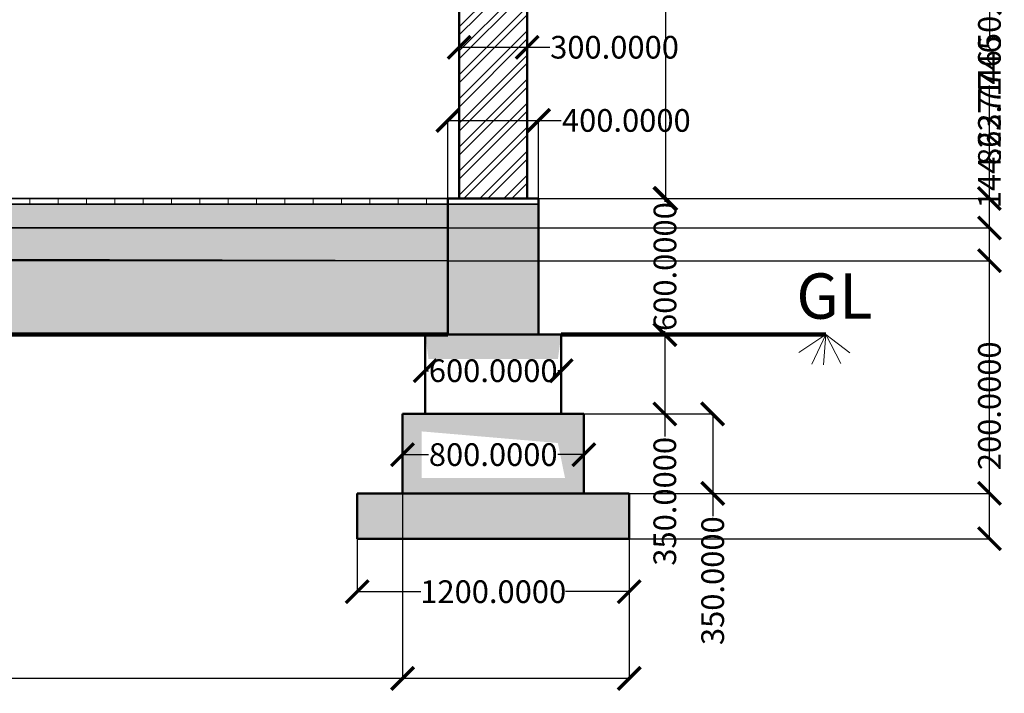
# Model space of a CAD drawing. Units: millimetres. Extents: x -4055 to 12299, y -682 to 5380.
# Tile 3 of 4: x 7955 to 12299, y -682 to 2289. Entities that reach past the tile are written whole.
import ezdxf

# ---------------------------------------------------------------- set-up
doc = ezdxf.new("R2010")
doc.units = ezdxf.units.MM
doc.header["$MEASUREMENT"] = 0
for name, color, linetype, lineweight in [('A-ANNO-DIMS', 2, 'Continuous', 18), ('A-ANNO-SYMB', 18, 'Continuous', 18), ('A-ANNO-TEXT', 7, 'Continuous', 18), ('A-FLOR', 7, 'Continuous', 35), ('A-FLOR-PATT', 8, 'Continuous', 13), ('A-WALL', 7, 'Continuous', 50), ('A-WALL-PATT', 8, 'Continuous', 13), ('gl', 18, 'Continuous', 120), ('S-FNDN', 7, 'Continuous', 50), ('S-FNDN-PATT', 8, 'Continuous', 13)]:
    doc.layers.add(name, color=color, linetype=linetype, lineweight=lineweight)
doc.styles.get("Standard").update_dxf_attribs({"font": 'arial.ttf'})
doc.dimstyles.get("Standard").update_dxf_attribs({"dimtxt": 100, "dimasz": 100, "dimexe": 0.18, "dimexo": 0.0625, "dimgap": 0.09, "dimtad": 0, "dimdec": 4, "dimzin": 0, "dimdsep": 46, "dimtxsty": 'Standard', "dimblk": 'ARCHTICK', "dimcen": 0.09, "dimclrd": 3, "dimclre": 6, "dimclrt": 1, "dimadec": 0, "dimazin": 0, "dimtfac": 1, "dimtdec": 4, "dimtofl": 0, "dimtmove": 0, "dimatfit": 3, "dimfxl": 1, "dimtolj": 1, "dimtzin": 0, "dimlwd": 30, "dimarcsym": 0})
pattern_1 = [(50, (0, 0), (71.72602, -6.2752), [7.5, -82.5]), (355, (0, 0), (-13.87513, 75.2192), [6, -66]), (100.45144, (5.98, -0.52), (57.8509, 68.944), [6.374, -70.1142]), (46.1842, (0, 20), (106.7241, -16.5519), [11.25, -123.75]), (96.6356, (8.89, 18.62), (93.4662, 97.4119), [9.561, -105.1714]), (351.1842, (0, 20), (93.4662, 97.4119), [9, -99]), (21, (10, 15), (59.6907, -40.2619), [7.5, -82.5]), (326, (10, 15), (24.33153, 72.515), [6, -66]), (71.45144, (14.974, 11.645), (84.02224, 32.2531), [6.374, -70.1142]), (37.5, (0, 0), (1.215986, 33.289385), [0, -65.2, 0, -67, 0, -66.25]), (7.5, (0, 0), (26.30695, 39.44117), [0, -38.2, 0, -63.7, 0, -25.25]), (327.5, (-22.3, 0), (53.382244, -2.25549), [0, -25, 0, -78, 0, -103.5]), (317.5, (-32.3, 0), (58.31862, 10.0105), [0, -32.5, 0, -51.8, 0, -73.5])]

# ---------------------------------------------------------------- blocks, each defined once
blk = doc.blocks.new('_ArchTick')
at = {"color": 0, "linetype": 'ByBlock', "const_width": 0.15}
blk.add_lwpolyline([(-0.5, -0.5), (0.5, 0.5)], dxfattribs=at)
blk = doc.blocks.new('*D2')
at = {"layer": 'A-ANNO-DIMS', "color": 0, "lineweight": -2, "transparency": 16777216}
for p, q in [((10194.1, 4500), (10805.3, 4500)), ((10194.1, 1500), (10805.3, 1500))]:
    blk.add_line(p, q, dxfattribs=at)
at = {"layer": 'A-ANNO-DIMS', "color": 0, "lineweight": 30, "transparency": 16777216}
for p, q in [((10805.2, 4500), (10805.2, 3324)), ((10805.2, 1500), (10805.2, 2676))]:
    blk.add_line(p, q, dxfattribs=at)
at = {"layer": 'Defpoints', "color": 0, "transparency": 16777216}
for p in [(10194, 4500), (10194, 1500), (10805.2, 1500)]:
    blk.add_point(p, dxfattribs=at)
at = {"layer": 'A-ANNO-DIMS', "color": 0, "lineweight": 30, "transparency": 16777216, "xscale": 100, "yscale": 100, "zscale": 100}
for p, rotation in [((10805.2, 4500), 90), ((10805.2, 1500), 270)]:
    blk.add_blockref('_ArchTick', p, dxfattribs=dict(at, rotation=rotation))
at = {"layer": 'A-ANNO-DIMS', "color": 0, "transparency": 16777216, "insert": (10805.2, 3000), "char_height": 100, "attachment_point": 5, "rotation": 90}
blk.add_mtext('\\A1;3000.0000', dxfattribs=at)
blk = doc.blocks.new('*D3')
at = {"layer": 'A-ANNO-DIMS', "color": 0, "lineweight": -2, "transparency": 16777216}
for p, q in [((10194.1, 1500), (10801.7, 1500)), ((10194.1, 900), (10801.7, 900))]:
    blk.add_line(p, q, dxfattribs=at)
at = {"layer": 'A-ANNO-DIMS', "color": 0, "lineweight": 30, "transparency": 16777216}
for p, q in [((10801.6, 1500), (10801.6, 1485.5)), ((10801.6, 900), (10801.6, 914.5))]:
    blk.add_line(p, q, dxfattribs=at)
at = {"layer": 'Defpoints', "color": 0, "transparency": 16777216}
for p in [(10194, 1500), (10194, 900), (10801.6, 900)]:
    blk.add_point(p, dxfattribs=at)
at = {"layer": 'A-ANNO-DIMS', "color": 0, "lineweight": 30, "transparency": 16777216, "xscale": 100, "yscale": 100, "zscale": 100}
for p, rotation in [((10801.6, 1500), 90), ((10801.6, 900), 270)]:
    blk.add_blockref('_ArchTick', p, dxfattribs=dict(at, rotation=rotation))
at = {"layer": 'A-ANNO-DIMS', "color": 0, "transparency": 16777216, "insert": (10801.6, 1200), "char_height": 100, "attachment_point": 5, "rotation": 90}
blk.add_mtext('\\A1;600.0000', dxfattribs=at)
blk = doc.blocks.new('*D4')
at = {"layer": 'A-ANNO-DIMS', "color": 0, "lineweight": -2, "transparency": 16777216}
for p, q in [((10344.1, 900), (10801.1, 900)), ((10344.1, 550), (10801.1, 550))]:
    blk.add_line(p, q, dxfattribs=at)
at = {"layer": 'A-ANNO-DIMS', "color": 0, "lineweight": 30, "transparency": 16777216}
for p, q in [((10800.9, 900), (10800.9, 550)), ((10800.9, 550), (10800.9, 450))]:
    blk.add_line(p, q, dxfattribs=at)
at = {"layer": 'Defpoints', "color": 0, "transparency": 16777216}
for p in [(10344, 900), (10344, 550), (10800.9, 550)]:
    blk.add_point(p, dxfattribs=at)
at = {"layer": 'A-ANNO-DIMS', "color": 0, "lineweight": 30, "transparency": 16777216, "xscale": 100, "yscale": 100, "zscale": 100}
for p, rotation in [((10800.9, 900), 90), ((10800.9, 550), 270)]:
    blk.add_blockref('_ArchTick', p, dxfattribs=dict(at, rotation=rotation))
at = {"layer": 'A-ANNO-DIMS', "color": 0, "transparency": 16777216, "insert": (10800.9, 164.8), "char_height": 100, "attachment_point": 5, "rotation": 90}
blk.add_mtext('\\A1;350.0000', dxfattribs=at)
blk = doc.blocks.new('*D5')
at = {"layer": 'A-ANNO-DIMS', "color": 0, "lineweight": -2, "transparency": 16777216}
for p, q in [((10444.1, 550), (11012.3, 550)), ((10444.1, 200), (11012.3, 200))]:
    blk.add_line(p, q, dxfattribs=at)
at = {"layer": 'A-ANNO-DIMS', "color": 0, "lineweight": 30, "transparency": 16777216}
for p, q in [((11012.1, 550), (11012.1, 200)), ((11012.1, 200), (11012.1, 100))]:
    blk.add_line(p, q, dxfattribs=at)
at = {"layer": 'Defpoints', "color": 0, "transparency": 16777216}
for p in [(10444, 550), (10444, 200), (11012.1, 200)]:
    blk.add_point(p, dxfattribs=at)
at = {"layer": 'A-ANNO-DIMS', "color": 0, "lineweight": 30, "transparency": 16777216, "xscale": 100, "yscale": 100, "zscale": 100}
for p, rotation in [((11012.1, 550), 90), ((11012.1, 200), 270)]:
    blk.add_blockref('_ArchTick', p, dxfattribs=dict(at, rotation=rotation))
at = {"layer": 'A-ANNO-DIMS', "color": 0, "transparency": 16777216, "insert": (11012.1, -185.2), "char_height": 100, "attachment_point": 5, "rotation": 90}
blk.add_mtext('\\A1;350.0000', dxfattribs=at)
blk = doc.blocks.new('*D6')
at = {"layer": 'A-ANNO-DIMS', "color": 0, "lineweight": -2, "transparency": 16777216}
for p, q in [((9444, -0.1), (9444, -233.8)), ((10644, -0.1), (10644, -233.8))]:
    blk.add_line(p, q, dxfattribs=at)
at = {"layer": 'A-ANNO-DIMS', "color": 0, "lineweight": 30, "transparency": 16777216}
for p, q in [((9444, -233.6), (9724.7, -233.6)), ((10644, -233.6), (10363.4, -233.6))]:
    blk.add_line(p, q, dxfattribs=at)
at = {"layer": 'Defpoints', "color": 0, "transparency": 16777216}
for p in [(9444, 0), (10644, 0), (10644, -233.6)]:
    blk.add_point(p, dxfattribs=at)
at = {"layer": 'A-ANNO-DIMS', "color": 0, "lineweight": 30, "transparency": 16777216, "xscale": 100, "yscale": 100, "zscale": 100, "rotation": 180}
blk.add_blockref('_ArchTick', (9444, -233.6), dxfattribs=at)
at = {"layer": 'A-ANNO-DIMS', "color": 0, "lineweight": 30, "transparency": 16777216, "xscale": 100, "yscale": 100, "zscale": 100}
blk.add_blockref('_ArchTick', (10644, -233.6), dxfattribs=at)
at = {"layer": 'A-ANNO-DIMS', "color": 0, "transparency": 16777216, "insert": (10044, -233.6), "char_height": 100, "attachment_point": 5}
blk.add_mtext('\\A1;1200.0000', dxfattribs=at)
blk = doc.blocks.new('*D7')
at = {"layer": 'A-ANNO-DIMS', "color": 0, "lineweight": -2, "transparency": 16777216}
for p, q in [((9644, 549.9), (9644, 370.6)), ((10444, 549.9), (10444, 370.6))]:
    blk.add_line(p, q, dxfattribs=at)
at = {"layer": 'A-ANNO-DIMS', "color": 0, "lineweight": 30, "transparency": 16777216}
for p, q in [((9644, 370.8), (9758.8, 370.8)), ((10444, 370.8), (10329.3, 370.8))]:
    blk.add_line(p, q, dxfattribs=at)
at = {"layer": 'Defpoints', "color": 0, "transparency": 16777216}
for p in [(9644, 550), (10444, 550), (10444, 370.8)]:
    blk.add_point(p, dxfattribs=at)
at = {"layer": 'A-ANNO-DIMS', "color": 0, "lineweight": 30, "transparency": 16777216, "xscale": 100, "yscale": 100, "zscale": 100, "rotation": 180}
blk.add_blockref('_ArchTick', (9644, 370.8), dxfattribs=at)
at = {"layer": 'A-ANNO-DIMS', "color": 0, "lineweight": 30, "transparency": 16777216, "xscale": 100, "yscale": 100, "zscale": 100}
blk.add_blockref('_ArchTick', (10444, 370.8), dxfattribs=at)
at = {"layer": 'A-ANNO-DIMS', "color": 0, "transparency": 16777216, "insert": (10044, 370.8), "char_height": 100, "attachment_point": 5}
blk.add_mtext('\\A1;800.0000', dxfattribs=at)
blk = doc.blocks.new('*D8')
at = {"layer": 'A-ANNO-DIMS', "color": 0, "lineweight": -2, "transparency": 16777216}
for p, q in [((9744, 899.9), (9744, 740.7)), ((10344, 899.9), (10344, 740.7))]:
    blk.add_line(p, q, dxfattribs=at)
at = {"layer": 'A-ANNO-DIMS', "color": 0, "lineweight": 30, "transparency": 16777216}
for p, q in [((9744, 740.8), (9758.6, 740.8)), ((10344, 740.8), (10329.5, 740.8))]:
    blk.add_line(p, q, dxfattribs=at)
at = {"layer": 'Defpoints', "color": 0, "transparency": 16777216}
for p in [(9744, 900), (10344, 900), (10344, 740.8)]:
    blk.add_point(p, dxfattribs=at)
at = {"layer": 'A-ANNO-DIMS', "color": 0, "lineweight": 30, "transparency": 16777216, "xscale": 100, "yscale": 100, "zscale": 100, "rotation": 180}
blk.add_blockref('_ArchTick', (9744, 740.8), dxfattribs=at)
at = {"layer": 'A-ANNO-DIMS', "color": 0, "lineweight": 30, "transparency": 16777216, "xscale": 100, "yscale": 100, "zscale": 100}
blk.add_blockref('_ArchTick', (10344, 740.8), dxfattribs=at)
at = {"layer": 'A-ANNO-DIMS', "color": 0, "transparency": 16777216, "insert": (10044, 740.8), "char_height": 100, "attachment_point": 5}
blk.add_mtext('\\A1;600.0000', dxfattribs=at)
blk = doc.blocks.new('*D9')
at = {"layer": 'A-ANNO-DIMS', "color": 0, "lineweight": -2, "transparency": 16777216}
for p, q in [((9844, 1500.1), (9844, 1844.7)), ((10244, 1500.1), (10244, 1844.7))]:
    blk.add_line(p, q, dxfattribs=at)
at = {"layer": 'A-ANNO-DIMS', "color": 0, "lineweight": 30, "transparency": 16777216}
for p, q in [((9844, 1844.5), (10244, 1844.5)), ((10244, 1844.5), (10344, 1844.5))]:
    blk.add_line(p, q, dxfattribs=at)
at = {"layer": 'Defpoints', "color": 0, "transparency": 16777216}
for p in [(10244, 1844.5), (9844, 1500), (10244, 1500)]:
    blk.add_point(p, dxfattribs=at)
at = {"layer": 'A-ANNO-DIMS', "color": 0, "lineweight": 30, "transparency": 16777216, "xscale": 100, "yscale": 100, "zscale": 100, "rotation": 180}
blk.add_blockref('_ArchTick', (9844, 1844.5), dxfattribs=at)
at = {"layer": 'A-ANNO-DIMS', "color": 0, "lineweight": 30, "transparency": 16777216, "xscale": 100, "yscale": 100, "zscale": 100}
blk.add_blockref('_ArchTick', (10244, 1844.5), dxfattribs=at)
at = {"layer": 'A-ANNO-DIMS', "color": 0, "transparency": 16777216, "insert": (10631.2, 1844.5), "char_height": 100, "attachment_point": 5}
blk.add_mtext('\\A1;400.0000', dxfattribs=at)
blk = doc.blocks.new('*D10')
at = {"layer": 'A-ANNO-DIMS', "color": 0, "lineweight": -2, "transparency": 16777216}
for p, q in [((9894, 1500.1), (9894, 2167.5)), ((10194, 1500.1), (10194, 2167.5))]:
    blk.add_line(p, q, dxfattribs=at)
at = {"layer": 'A-ANNO-DIMS', "color": 0, "lineweight": 30, "transparency": 16777216}
for p, q in [((9894, 2167.3), (10194, 2167.3)), ((10194, 2167.3), (10294, 2167.3))]:
    blk.add_line(p, q, dxfattribs=at)
at = {"layer": 'Defpoints', "color": 0, "transparency": 16777216}
for p in [(10194, 2167.3), (9894, 1500), (10194, 1500)]:
    blk.add_point(p, dxfattribs=at)
at = {"layer": 'A-ANNO-DIMS', "color": 0, "lineweight": 30, "transparency": 16777216, "xscale": 100, "yscale": 100, "zscale": 100, "rotation": 180}
blk.add_blockref('_ArchTick', (9894, 2167.3), dxfattribs=at)
at = {"layer": 'A-ANNO-DIMS', "color": 0, "lineweight": 30, "transparency": 16777216, "xscale": 100, "yscale": 100, "zscale": 100}
blk.add_blockref('_ArchTick', (10194, 2167.3), dxfattribs=at)
at = {"layer": 'A-ANNO-DIMS', "color": 0, "transparency": 16777216, "insert": (10579.2, 2167.3), "char_height": 100, "attachment_point": 5}
blk.add_mtext('\\A1;300.0000', dxfattribs=at)
blk = doc.blocks.new('FNDN-STEPPED-1200')
for p, q in [((-200, 900), (-200, 1500)), ((-200, 1500), (200, 1500)), ((200, 1500), (200, 900)), ((-300, 550), (-300, 900)), ((-300, 900), (300, 900)), ((300, 900), (300, 550)), ((-400, 200), (-400, 550)), ((-400, 550), (400, 550)), ((400, 550), (400, 200)), ((600, 200), (-600, 200)), ((-600, 200), (-600, 0)), ((600, 0), (600, 200)), ((-600, 0), (600, 0))]:
    blk.add_line(p, q)
blk = doc.blocks.new('*D18')
at = {"layer": 'A-ANNO-DIMS', "color": 6, "lineweight": -2, "transparency": 16777216}
for p, q in [((0, -0.1), (0, -616.4)), ((10644, -0.1), (10644, -616.4))]:
    blk.add_line(p, q, dxfattribs=at)
at = {"layer": 'A-ANNO-DIMS', "color": 3, "lineweight": 30, "transparency": 16777216}
for p, q in [((0, -616.2), (4963.8, -616.2)), ((10644, -616.2), (5680.2, -616.2))]:
    blk.add_line(p, q, dxfattribs=at)
at = {"layer": 'Defpoints', "color": 0, "transparency": 16777216}
for p in [(0, 0), (10644, 0), (10644, -616.2)]:
    blk.add_point(p, dxfattribs=at)
at = {"layer": 'A-ANNO-DIMS', "color": 3, "lineweight": 30, "transparency": 16777216, "xscale": 100, "yscale": 100, "zscale": 100, "rotation": 180}
blk.add_blockref('_ArchTick', (0, -616.2), dxfattribs=at)
at = {"layer": 'A-ANNO-DIMS', "color": 3, "lineweight": 30, "transparency": 16777216, "xscale": 100, "yscale": 100, "zscale": 100}
blk.add_blockref('_ArchTick', (10644, -616.2), dxfattribs=at)
at = {"layer": 'A-ANNO-DIMS', "color": 1, "transparency": 16777216, "insert": (5322, -616.2), "char_height": 100, "attachment_point": 5}
blk.add_mtext('\\A1;10644.0310', dxfattribs=at)
blk = doc.blocks.new('*D19')
at = {"layer": 'A-ANNO-DIMS', "color": 6, "lineweight": -2, "transparency": 16777216}
for p, q in [((10394.1, 4650), (12233.2, 4650)), ((10644.1, 0), (12233.2, 0))]:
    blk.add_line(p, q, dxfattribs=at)
at = {"layer": 'A-ANNO-DIMS', "color": 3, "lineweight": 30, "transparency": 16777216}
for p, q in [((12233, 4650), (12233, 2651)), ((12233, 0), (12233, 1999))]:
    blk.add_line(p, q, dxfattribs=at)
at = {"layer": 'Defpoints', "color": 0, "transparency": 16777216}
for p in [(10394, 4650), (12233, 4650), (10644, 0)]:
    blk.add_point(p, dxfattribs=at)
at = {"layer": 'A-ANNO-DIMS', "color": 3, "lineweight": 30, "transparency": 16777216, "xscale": 100, "yscale": 100, "zscale": 100}
for p, rotation in [((12233, 4650), 90), ((12233, 0), 270)]:
    blk.add_blockref('_ArchTick', p, dxfattribs=dict(at, rotation=rotation))
at = {"layer": 'A-ANNO-DIMS', "color": 1, "transparency": 16777216, "insert": (12233, 2325), "char_height": 100, "attachment_point": 5, "rotation": 90}
blk.add_mtext('\\A1;4650.0000', dxfattribs=at)
blk = doc.blocks.new('*D21')
at = {"layer": 'A-ANNO-DIMS', "color": 6, "lineweight": -2, "transparency": 16777216}
for p, q in [((5444.6, 549.9), (5444.6, -616.4)), ((9644, 549.9), (9644, -616.4))]:
    blk.add_line(p, q, dxfattribs=at)
at = {"layer": 'A-ANNO-DIMS', "color": 3, "lineweight": 30, "transparency": 16777216}
for p, q in [((5444.6, -616.2), (7218.3, -616.2)), ((9644, -616.2), (7870.4, -616.2))]:
    blk.add_line(p, q, dxfattribs=at)
at = {"layer": 'Defpoints', "color": 0, "transparency": 16777216}
for p in [(5444.6, 550), (9644, 550), (9644, -616.2)]:
    blk.add_point(p, dxfattribs=at)
at = {"layer": 'A-ANNO-DIMS', "color": 3, "lineweight": 30, "transparency": 16777216, "xscale": 100, "yscale": 100, "zscale": 100, "rotation": 180}
blk.add_blockref('_ArchTick', (5444.6, -616.2), dxfattribs=at)
at = {"layer": 'A-ANNO-DIMS', "color": 3, "lineweight": 30, "transparency": 16777216, "xscale": 100, "yscale": 100, "zscale": 100}
blk.add_blockref('_ArchTick', (9644, -616.2), dxfattribs=at)
at = {"layer": 'A-ANNO-DIMS', "color": 1, "transparency": 16777216, "insert": (7544.3, -616.2), "char_height": 100, "attachment_point": 5}
blk.add_mtext('\\A1;4199.4230', dxfattribs=at)
blk = doc.blocks.new('*D30')
at = {"layer": 'A-ANNO-DIMS', "color": 3, "lineweight": 30, "transparency": 16777216}
for p, q in [((12233, 200), (12233, 300)), ((12233, 0), (12233, 200))]:
    blk.add_line(p, q, dxfattribs=at)
at = {"layer": 'A-ANNO-DIMS', "color": 6, "lineweight": -2, "transparency": 16777216}
for p, q in [((10644.1, 200), (12233.2, 200)), ((10644.1, 0), (12233.2, 0))]:
    blk.add_line(p, q, dxfattribs=at)
at = {"layer": 'Defpoints', "color": 0, "transparency": 16777216}
for p in [(10644, 200), (12233, 200), (10644, 0)]:
    blk.add_point(p, dxfattribs=at)
at = {"layer": 'A-ANNO-DIMS', "color": 3, "lineweight": 30, "transparency": 16777216, "xscale": 100, "yscale": 100, "zscale": 100}
for p, rotation in [((12233, 200), 90), ((12233, 0), 270)]:
    blk.add_blockref('_ArchTick', p, dxfattribs=dict(at, rotation=rotation))
at = {"layer": 'A-ANNO-DIMS', "color": 1, "transparency": 16777216, "insert": (12233, 586), "char_height": 100, "attachment_point": 5, "rotation": 90}
blk.add_mtext('\\A1;200.0000', dxfattribs=at)
blk = doc.blocks.new('*D31')
at = {"layer": 'A-ANNO-DIMS', "color": 3, "lineweight": 30, "transparency": 16777216}
for p, q in [((-1060.6, 1226), (-1060.6, 1326)), ((-1060.6, 900), (-1060.6, 1226))]:
    blk.add_line(p, q, dxfattribs=at)
at = {"layer": 'A-ANNO-DIMS', "color": 6, "lineweight": -2, "transparency": 16777216}
for p, q in [((9844, 1226), (-1060.8, 1226)), ((9844, 900), (-1060.8, 900))]:
    blk.add_line(p, q, dxfattribs=at)
at = {"layer": 'Defpoints', "color": 0, "transparency": 16777216}
for p in [(-1060.6, 1226), (9844, 1226), (9844, 900)]:
    blk.add_point(p, dxfattribs=at)
at = {"layer": 'A-ANNO-DIMS', "color": 3, "lineweight": 30, "transparency": 16777216, "xscale": 100, "yscale": 100, "zscale": 100}
for p, rotation in [((-1060.6, 1226), 90), ((-1060.6, 900), 270)]:
    blk.add_blockref('_ArchTick', p, dxfattribs=dict(at, rotation=rotation))
at = {"layer": 'A-ANNO-DIMS', "color": 1, "transparency": 16777216, "insert": (-1060.6, 1611.4), "char_height": 100, "attachment_point": 5, "rotation": 90}
blk.add_mtext('\\A1;326.0158', dxfattribs=at)
blk = doc.blocks.new('*D32')
at = {"layer": 'A-ANNO-DIMS', "color": 3, "lineweight": 30, "transparency": 16777216}
for p, q in [((12233, 1370.2), (12233, 1470.2)), ((12233, 1226), (12233, 1370.2))]:
    blk.add_line(p, q, dxfattribs=at)
at = {"layer": 'A-ANNO-DIMS', "color": 6, "lineweight": -2, "transparency": 16777216}
for p, q in [((9844.1, 1370.2), (12233.2, 1370.2)), ((9844.1, 1226), (12233.2, 1226))]:
    blk.add_line(p, q, dxfattribs=at)
at = {"layer": 'Defpoints', "color": 0, "transparency": 16777216}
for p in [(9844, 1370.2), (12233, 1370.2), (9844, 1226)]:
    blk.add_point(p, dxfattribs=at)
at = {"layer": 'A-ANNO-DIMS', "color": 3, "lineweight": 30, "transparency": 16777216, "xscale": 100, "yscale": 100, "zscale": 100}
for p, rotation in [((12233, 1370.2), 90), ((12233, 1226), 270)]:
    blk.add_blockref('_ArchTick', p, dxfattribs=dict(at, rotation=rotation))
at = {"layer": 'A-ANNO-DIMS', "color": 1, "transparency": 16777216, "insert": (12233, 1741.2), "char_height": 100, "attachment_point": 5, "rotation": 90}
blk.add_mtext('\\A1;144.2271', dxfattribs=at)
blk = doc.blocks.new('*D33')
at = {"layer": 'A-ANNO-DIMS', "color": 3, "lineweight": 30, "transparency": 16777216}
for p, q in [((-1060.6, 1500), (-1060.6, 1600)), ((-1060.6, 1370.2), (-1060.6, 1500))]:
    blk.add_line(p, q, dxfattribs=at)
at = {"layer": 'A-ANNO-DIMS', "color": 6, "lineweight": -2, "transparency": 16777216}
for p, q in [((9844, 1500), (-1060.8, 1500)), ((9844, 1370.2), (-1060.8, 1370.2))]:
    blk.add_line(p, q, dxfattribs=at)
at = {"layer": 'Defpoints', "color": 0, "transparency": 16777216}
for p in [(-1060.6, 1500), (9844, 1500), (9844, 1370.2)]:
    blk.add_point(p, dxfattribs=at)
at = {"layer": 'A-ANNO-DIMS', "color": 3, "lineweight": 30, "transparency": 16777216, "xscale": 100, "yscale": 100, "zscale": 100}
for p, rotation in [((-1060.6, 1500), 90), ((-1060.6, 1370.2), 270)]:
    blk.add_blockref('_ArchTick', p, dxfattribs=dict(at, rotation=rotation))
at = {"layer": 'A-ANNO-DIMS', "color": 1, "transparency": 16777216, "insert": (-1060.6, 1871), "char_height": 100, "attachment_point": 5, "rotation": 90}
blk.add_mtext('\\A1;129.7571', dxfattribs=at)
blk = doc.blocks.new('*D34')
at = {"layer": 'A-ANNO-DIMS', "color": 6, "lineweight": -2, "transparency": 16777216}
for p, q in [((6374.7, 2363.8), (12233.2, 2363.8)), ((6374.7, 1500), (12233.2, 1500))]:
    blk.add_line(p, q, dxfattribs=at)
at = {"layer": 'A-ANNO-DIMS', "color": 3, "lineweight": 30, "transparency": 16777216}
for p, q in [((12233, 2363.8), (12233, 2217.3)), ((12233, 1500), (12233, 1646.5))]:
    blk.add_line(p, q, dxfattribs=at)
at = {"layer": 'Defpoints', "color": 0, "transparency": 16777216}
for p in [(6374.6, 2363.8), (12233, 2363.8), (6374.6, 1500)]:
    blk.add_point(p, dxfattribs=at)
at = {"layer": 'A-ANNO-DIMS', "color": 3, "lineweight": 30, "transparency": 16777216, "xscale": 100, "yscale": 100, "zscale": 100}
for p, rotation in [((12233, 2363.8), 90), ((12233, 1500), 270)]:
    blk.add_blockref('_ArchTick', p, dxfattribs=dict(at, rotation=rotation))
at = {"layer": 'A-ANNO-DIMS', "color": 1, "transparency": 16777216, "insert": (12233, 1931.9), "char_height": 100, "attachment_point": 5, "rotation": 90}
blk.add_mtext('\\A1;863.7746', dxfattribs=at)

msp = doc.modelspace()

# ---------------------------------------------------------------- hatches: boundary and pattern name
at = {"layer": 'A-FLOR-PATT'}
h = msp.add_hatch(dxfattribs=at)
h.set_pattern_fill('NET', color=256, scale=1000)
h.paths.add_polyline_path([(3028.64487, 1500), (1878.64487, 1500), (800, 1500), (800, 1475), (3028.64487, 1475)])
h.paths.add_polyline_path([(4844.60797, 1500), (3428.64487, 1500), (3428.64487, 1475), (4844.60797, 1475)])
h.paths.add_polyline_path([(9844.03102, 1500), (5244.60797, 1500), (5244.60797, 1475), (9844.03102, 1475)])
h = msp.add_hatch(dxfattribs=at)
h.set_pattern_fill('AR-SAND', color=256, scale=10)
h.paths.add_polyline_path([(9844.03102, 1475), (5244.60797, 1475), (5244.60797, 1372.3308), (9844.03102, 1370.24292)])
h.paths.add_polyline_path([(4844.60797, 1475), (3428.64487, 1475), (3428.64487, 1373.15514), (4844.60797, 1372.51237)])
h.paths.add_polyline_path([(3428.64487, 1475), (3028.64487, 1475), (3028.64487, 1373.33672), (3428.64487, 1373.15514)])
h.paths.add_polyline_path([(3028.64487, 1475), (800, 1475), (800, 1374.34839), (3028.64487, 1373.33672)])
h = msp.add_hatch(dxfattribs=at)
h.set_pattern_fill('AR-CONC', color=256, scale=10)
h.set_pattern_definition(pattern_1)
h.paths.add_polyline_path([(4844.60797, 1372.51237), (3428.64487, 1373.15514), (3428.64487, 1242.30842), (4844.60797, 1238.71243)])
h.paths.add_polyline_path([(9844.03102, 1370.24292), (5244.60797, 1372.3308), (5244.60797, 1237.69658), (9844.03102, 1226.01584)])
h.paths.add_polyline_path([(3028.64487, 1373.33672), (800, 1374.34839), (800, 1248.98416), (3028.64487, 1243.32427)])
h = msp.add_hatch(dxfattribs=at)
h.set_pattern_fill('GRAVEL', color=256, scale=300)
h.paths.add_polyline_path([(4844.60797, 1238.71243), (3428.64487, 1242.30842), (3428.64487, 900), (4844.60797, 900)])
h.paths.add_polyline_path([(9844.03102, 1226.01584), (5244.60797, 1237.69658), (5244.60797, 900), (9844.03102, 900)])
h.paths.add_polyline_path([(3028.64487, 1243.32427), (800, 1248.98416), (800, 900), (3028.64487, 900)])
at = {"layer": 'A-WALL-PATT'}
h = msp.add_hatch(dxfattribs=at)
h.set_pattern_fill('ANSI32', color=256, scale=200)
h.paths.add_polyline_path([(750, 3719.22559), (450, 3719.22559), (450, 1500), (750, 1500)])
h.paths.add_polyline_path([(3378.64487, 4500), (3078.64487, 4500), (3078.64487, 1500), (3378.64487, 1500)])
h.paths.add_polyline_path([(5194.60797, 4500), (4894.60797, 4500), (4894.60797, 1500), (5194.60797, 1500), (5194.60797, 3600)])
h.paths.add_polyline_path([(750, 4500), (450, 4500), (450, 4209.88871), (750, 4209.88871)])
h.paths.add_polyline_path([(10194.03102, 4500), (9894.03102, 4500), (9894.03102, 1500), (10194.03102, 1500)])
at = {"layer": 'S-FNDN-PATT'}
h = msp.add_hatch(dxfattribs=at)
h.set_pattern_fill('ANSI33', color=256, scale=400)
h.paths.add_polyline_path([(1000, 550), (200, 550), (200, 200), (1000, 200)])
h.paths.add_polyline_path([(800, 1475), (750, 1475), (400, 1475), (400, 900), (800, 900)])
h.paths.add_polyline_path([(900, 900), (300, 900), (300, 550), (900, 550)])
h.paths.add_polyline_path([(3528.64487, 900), (2928.64487, 900), (2928.64487, 550), (3183.63873, 549.73878), (3186.06833, 624.99556), (3283.2525, 501.18603), (3300.25973, 554.59402), (3528.64487, 550)])
h.paths.add_polyline_path([(3428.64487, 1242.30842), (3028.64487, 1243.32427), (3028.64487, 900), (3428.64487, 900)])
h.paths.add_polyline_path([(3428.64487, 1373.15514), (3028.64487, 1373.33672), (3028.64487, 1243.32427), (3428.64487, 1242.30842)])
h.paths.add_polyline_path([(5244.60797, 1372.3308), (4844.60797, 1372.51237), (4844.60797, 1238.71243), (5244.60797, 1237.69658)])
h.paths.add_polyline_path([(5244.60797, 1237.69658), (4844.60797, 1238.71243), (4844.60797, 900), (5244.60797, 900)])
h.paths.add_polyline_path([(5244.60797, 1475), (4844.60797, 1475), (4844.60797, 1372.51237), (5244.60797, 1372.3308)])
h.paths.add_polyline_path([(5444.60797, 550), (4644.60797, 550), (4644.60797, 200), (5444.60797, 200)])
h.paths.add_polyline_path([(5344.60797, 900), (4744.60797, 900), (4744.60797, 550), (5344.60797, 550)])
h.paths.add_polyline_path([(10344.03102, 900), (9744.03102, 900), (9758.66267, 791.89949), (10329.39937, 791.89949)])
h.paths.add_polyline_path([(10244.03102, 1475), (9894.03102, 1475), (9844.03102, 1475), (9844.03102, 900), (10244.03102, 900)])
h.paths.add_polyline_path([(10444.03102, 550), (9644.03102, 550), (9644.03102, 200), (10444.03102, 200)])
h.paths.add_polyline_path([(9728.20564, 267.06671), (10360.87959, 267.06671), (10329.19473, 421.87571), (9728.20564, 473.13765)], flags=16)
h = msp.add_hatch(dxfattribs=at)
h.set_pattern_fill('AR-CONC', color=256, scale=10)
h.set_pattern_definition(pattern_1)
h.paths.add_polyline_path([(1200, 200), (0, 200), (0, 0), (1200, 0)])
h.paths.add_polyline_path([(5644.60797, 200), (4444.60797, 200), (4444.60797, 0), (5644.60797, 0)])
h.paths.add_polyline_path([(10644.03102, 200), (9444.03102, 200), (9444.03102, 0), (10644.03102, 0)])

# ---------------------------------------------------------------- linework, layer by layer
at = {"layer": 'A-ANNO-SYMB'}
for p, q in [((11511.0228, 900), (11391.87547, 821.56859)), ((11391.87547, 821.56859), (11511.0228, 900)), ((11511.0228, 900), (11449.40051, 769.31531)), ((11449.40051, 769.31531), (11511.0228, 900)), ((11511.0228, 900), (11449.40051, 769.31531)), ((11449.40051, 769.31531), (11511.0228, 900)), ((11511.0228, 900), (11501.69619, 766.70266)), ((11501.69619, 766.70266), (11511.0228, 900)), ((11511.0228, 900), (11616.74644, 818.95587)), ((11616.74644, 818.95587), (11511.0228, 900)), ((11511.0228, 900), (11577.52477, 771.92796)), ((11577.52477, 771.92796), (11511.0228, 900)), ((11511.0228, 900), (11616.74644, 818.95587))]:
    msp.add_line(p, q, dxfattribs=at)
at = {"layer": 'A-FLOR'}
for p, q in [((800, 1500), (9844.03102, 1500)), ((10244.03102, 1500), (10244.03102, 1475)), ((9894.03102, 1475), (750, 1475)), ((10244.03102, 1475), (9894.03102, 1475)), ((800, 1374.34839), (9844.03102, 1370.24292)), ((800, 1248.98416), (9844.03102, 1226.01584))]:
    msp.add_line(p, q, dxfattribs=at)
at = {"layer": 'A-WALL'}
for p, q in [((9894.03102, 1500), (9894.03102, 4500)), ((10194.03102, 4500), (10194.03102, 1500))]:
    msp.add_line(p, q, dxfattribs=at)
at = {"layer": 'gl'}
for p, q in [((800, 900), (9844.03102, 900)), ((10344.03102, 900), (11511.0228, 900))]:
    msp.add_line(p, q, dxfattribs=at)

# ---------------------------------------------------------------- block references
at = {"layer": 'S-FNDN'}
msp.add_blockref('FNDN-STEPPED-1200', (10044.03102, 0), dxfattribs=at)

# ---------------------------------------------------------------- texts
at = {"layer": 'A-ANNO-TEXT', "insert": (11381.13672, 1170.0828), "char_height": 200, "attachment_point": 1}
msp.add_mtext_dynamic_manual_height_columns('GL', width=303.3143068, gutter_width=1, heights=[0], dxfattribs=at)

# ---------------------------------------------------------------- dimensions: what is measured, and where the dimension line sits
at = {"layer": 'A-ANNO-DIMS'}
for base, p1, p2, override, picture, middle in [((12232.99644, 4650), (10644.03102, 0), (10394.03102, 4650), {"dimdec": 4, "dimlfac": 1, "dimrnd": 0, "dimzin": 0, "dimdsep": 46, "dimlunit": 2}, '*D19', (12232.99644, 2325)), ((10805.16529, 1500), (10194.03102, 4500), (10194.03102, 1500), {"dimclrd": 0, "dimclre": 0, "dimclrt": 0}, '*D2', (10805.16529, 3000)), ((12232.99644, 2363.77463), (6374.60797, 1500), (6374.60797, 2363.77463), {"dimdec": 4, "dimlfac": 1, "dimrnd": 0, "dimzin": 0, "dimdsep": 46, "dimlunit": 2}, '*D34', (12232.99644, 1931.88731)), ((-1060.61411, 1500), (9844.03102, 1370.24292), (9844.03102, 1500), {"dimdec": 4, "dimlfac": 1, "dimrnd": 0, "dimzin": 0, "dimdsep": 46, "dimlunit": 2}, '*D33', (-1060.61411, 1870.99723)), ((12232.99644, 1370.24292), (9844.03102, 1226.01584), (9844.03102, 1370.24292), {"dimdec": 4, "dimlfac": 1, "dimrnd": 0, "dimzin": 0, "dimdsep": 46, "dimlunit": 2}, '*D32', (12232.99644, 1741.24015)), ((-1060.61411, 1226.01584), (9844.03102, 900), (9844.03102, 1226.01584), {"dimdec": 4, "dimlfac": 1, "dimrnd": 0, "dimzin": 0, "dimdsep": 46, "dimlunit": 2}, '*D31', (-1060.61411, 1611.44009)), ((10801.5569, 900), (10194.03102, 1500), (10194.03102, 900), {"dimclrd": 0, "dimclre": 0, "dimclrt": 0}, '*D3', (10801.5569, 1200)), ((10800.92988, 550), (10344.03102, 900), (10344.03102, 550), {"dimclrd": 0, "dimclre": 0, "dimclrt": 0}, '*D4', (10800.92988, 164.84861)), ((12232.99644, 200), (10644.03102, 0), (10644.03102, 200), {"dimdec": 4, "dimlfac": 1, "dimrnd": 0, "dimzin": 0, "dimdsep": 46, "dimlunit": 2}, '*D30', (12232.99644, 586.03816)), ((11012.14447, 200), (10444.03102, 550), (10444.03102, 200), {"dimclrd": 0, "dimclre": 0, "dimclrt": 0}, '*D5', (11012.14447, -185.15139))]:
    dim = msp.add_linear_dim(base=base, p1=p1, p2=p2, angle=90, dimstyle='Standard', override=override, dxfattribs=at)
    dim.commit()
    dim.dimension.update_dxf_attribs({"geometry": picture, "text_midpoint": middle})
for base, p1, p2, override, picture, middle in [((10194.03102, 2167.29345), (9894.03102, 1500), (10194.03102, 1500), {"dimclrd": 0, "dimclre": 0, "dimclrt": 0}, '*D10', (10579.18241, 2167.29345)), ((10344.03102, 740.84219), (9744.03102, 900), (10344.03102, 900), {"dimclrd": 0, "dimclre": 0, "dimclrt": 0}, '*D8', (10044.03102, 740.84219)), ((9644.031019, -616.25), (5444.607971, 550), (9644.031019, 550), {"dimdec": 4, "dimlfac": 1, "dimrnd": 0, "dimzin": 0, "dimdsep": 46, "dimlunit": 2}, '*D21', (7544.319495, -616.25)), ((10444.03102, 370.81841), (9644.03102, 550), (10444.03102, 550), {"dimclrd": 0, "dimclre": 0, "dimclrt": 0}, '*D7', (10044.03102, 370.81841)), ((10644.03102, -616.25), (0, 0), (10644.03102, 0), {"dimdec": 4, "dimlfac": 1, "dimrnd": 0, "dimzin": 0, "dimdsep": 46, "dimlunit": 2}, '*D18', (5322.01551, -616.25)), ((10644.03102, -233.64793), (9444.03102, 0), (10644.03102, 0), {"dimclrd": 0, "dimclre": 0, "dimclrt": 0}, '*D6', (10044.03102, -233.64793))]:
    dim = msp.add_linear_dim(base=base, p1=p1, p2=p2, dimstyle='Standard', override=override, dxfattribs=at)
    dim.commit()
    dim.dimension.update_dxf_attribs({"geometry": picture, "text_midpoint": middle})
dim = msp.add_linear_dim(base=(10244.03102, 1844.50015), p1=(9844.03102, 1500), p2=(10244.03102, 1500), angle=0, dimstyle='Standard', override={"dimclrd": 0, "dimclre": 0, "dimclrt": 0}, dxfattribs=at)
dim.commit()
dim.dimension.update_dxf_attribs({"geometry": '*D9', "text_midpoint": (10631.2288, 1844.50015), "dimtype": 161})

doc.saveas('drawing.dxf')
